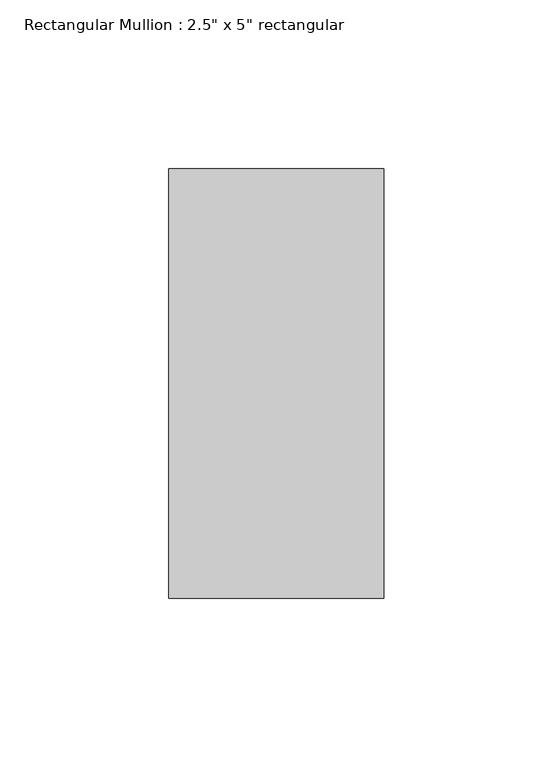
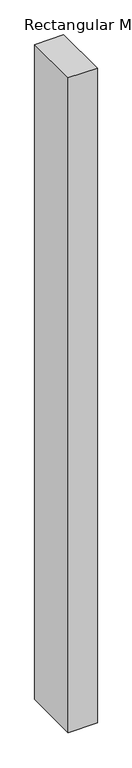
"""IFC4 building model written with IfcOpenShell, lengths in millimetres: member geometry."""

from ifc_helpers import new_model, si_unit, frame, origin, place, context, project, spatial, polyline, outline, extrude, source, transform, mapped, element, save


def member_83289212(model_context):
    return source(origin(), model_context, "Body", "SweptSolid", [
        extrude(outline(polyline([(0.0, 63.5), (0.0, -63.5), (-63.5, -63.5), (-63.5, 63.5), (0.0, 63.5)])), frame((0.0, 0.0, -1512.8617517), z_axis=(0.0, 0.0, 1.0), x_axis=(1.0, 0.0, 0.0)), (0.0, 0.0, 1.0), 1512.8617517),
    ])


if __name__ == "__main__":
    model = new_model("IFC4")
    model_context = context("Model", 3, world=origin())
    ifc_project = project(units=[si_unit("LENGTHUNIT", "METRE", prefix="MILLI")], contexts=[model_context])
    site = spatial("IfcSite", under=ifc_project)
    building = spatial("IfcBuilding", under=site)
    placement = place(None, origin())
    member_shape = member_83289212(model_context)
    element("IfcMember", 1, ObjectType="Rectangular Mullion : 2.5\" x 5\" rectangular", at=placement, inside=building, context=model_context, shape_type="MappedRepresentation", body=[
        mapped(member_shape, transform((0.0, 0.0, 0.0), x_axis=(1.0, 0.0, 0.0), y_axis=(0.0, 1.0, 0.0), z_axis=(0.0, 0.0, 1.0))),
    ])
    save(model, "model.ifc")

# Revit data of these elements
# Type "Rectangular Mullion : 2.5\" x 5\" rectangular"
#   built-in parameter 1007304 = 0.416667 (stored number, unit not read)
#   built-in parameter 1007301 = 0.104167 (stored number, unit not read)
#   built-in parameter 1007300 = 0.104167 (stored number, unit not read)
# Element 1 (IfcMember, "Rectangular Mullion : 2.5\" x 5\" rectangular")
#   Materials on its faces: "Aluminum"
# Materials
#   "Aluminum": class "Metal", colour RGB 247 247 247, transparency 0, Description = "Aluminum 6061", Cost = 0
